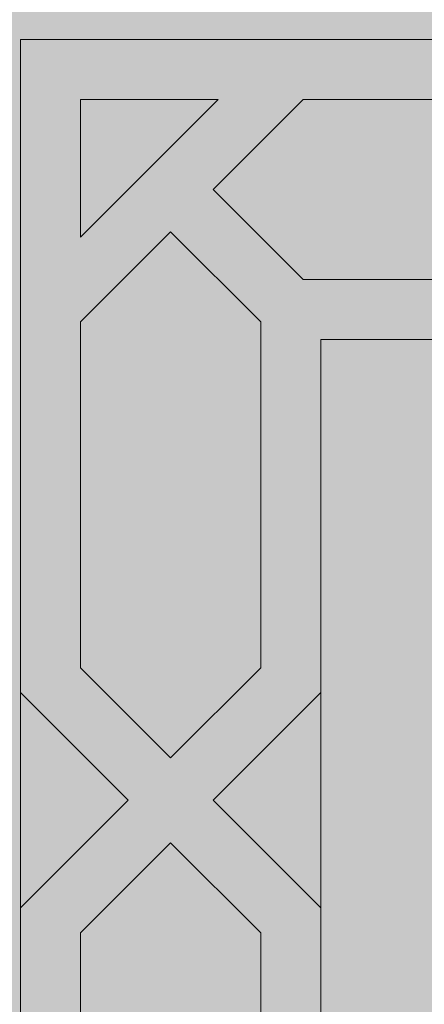
# Model space of a CAD drawing. Units: inches. Extents: x 844 to 2234, y 346 to 1084.
# Tile 81 of 93: x 1997.478 to 1999.197, y 708.742 to 712.926. Entities that reach past the tile are written whole.
import ezdxf

# ---------------------------------------------------------------- set-up
doc = ezdxf.new("R2010")
doc.units = ezdxf.units.IN
doc.header["$MEASUREMENT"] = 0
for name, color, linetype, lineweight in [('A-ANNO-DIMS', 2, 'Continuous', 18), ('furniture', 8, 'Continuous', 18), ('RA-AP-01$0$INT', 35, 'Continuous', 5)]:
    doc.layers.add(name, color=color, linetype=linetype, lineweight=lineweight)
doc.layers.add('RA-AP-01$0$FURN', color=3, linetype='Continuous')
doc.styles.get("Standard").update_dxf_attribs({"font": 'arial.ttf'})
doc.dimstyles.get("Standard").update_dxf_attribs({"dimtxt": 6, "dimasz": 3, "dimexe": 0.18, "dimexo": 0.0625, "dimgap": 0.09, "dimtad": 0, "dimtih": 1, "dimtoh": 1, "dimdec": 1, "dimzin": 0, "dimdsep": 46, "dimlunit": 3, "dimtxsty": 'Standard', "dimblk": 'ARCHTICK', "dimcen": 0.09, "dimadec": 0, "dimazin": 0, "dimtfac": 1, "dimtdec": 1, "dimtofl": 0, "dimtmove": 0, "dimatfit": 3, "dimfxl": 1, "dimtolj": 1, "dimtzin": 0, "dimarcsym": 0})

# ---------------------------------------------------------------- blocks, each defined once
blk = doc.blocks.new('A$C18D01794')
at = {"layer": 'RA-AP-01$0$INT'}
h = blk.add_hatch(color=256, dxfattribs=at)
h.paths.add_polyline_path([(4.355206456958071, -6.156712009588037), (4.355206456958071, -8.056712009588038), (5.455206456958072, -8.056712009588038), (5.455206456958072, -6.156712009588037)])
h.paths.add_polyline_path([(4.405206456958072, -8.006712009588039), (4.405206456958072, -6.206712009588038), (5.405206456958072, -6.206712009588038), (5.405206456958072, -8.006712009588039)], flags=16)
h = blk.add_hatch(color=256, dxfattribs=at)
h.paths.add_polyline_path([(4.505206456958071, -7.585498806127123), (4.46934859260189, -7.549640941759413), (4.505206456958071, -7.513783077414768), (4.505206456958071, -7.381963272220687), (4.469348592616735, -7.346105407867824), (4.505206456958071, -7.310247543514964), (4.505206456958071, -7.178427738324996), (4.469348592586679, -7.142569873965138), (4.505206456952245, -7.106712009588038), (4.476922185709333, -7.106712009588038), (4.455206456960671, -7.128427738343681), (4.433490728198047, -7.106712009588038), (4.405206456946033, -7.106712009588036), (4.441064321339216, -7.142569873969684), (4.40520645695807, -7.178427738362358), (4.405206456958072, -7.310247543472698), (4.441064321364728, -7.346105407867826), (4.40520645695807, -7.381963272262947), (4.40520645695807, -7.513783077378263), (4.441064321354429, -7.549640941786153), (4.405206456958072, -7.585498806170974), (4.405206456958072, -7.717318611286652), (4.441064321333084, -7.753176475673194), (4.405206456958072, -7.789034340036673), (4.405206456958072, -8.006712009588039), (4.644348592588106, -8.006712009588039), (4.680206456964639, -7.970854145211967), (4.716064321341165, -8.006712009588039), (4.869348592586113, -8.006712009588039), (4.905206456964143, -7.970854145210465), (4.941064321342174, -8.006712009588039), (5.094348592587118, -8.006712009588037), (5.130206456963649, -7.970854145211967), (5.166064321340178, -8.006712009588039), (5.405206456958072, -8.006712009588039), (5.405206456958072, -7.789034340024526), (5.369348592595202, -7.753176475673196), (5.40520645695807, -7.717318611298797), (5.40520645695807, -7.585498806158829), (5.369348592573859, -7.549640941786151), (5.40520645695807, -7.51378307739041), (5.40520645695807, -7.381963272250803), (5.36934859256356, -7.346105407867824), (5.405206456958072, -7.310247543484846), (5.405206456958072, -7.178427738350217), (5.369348592589068, -7.142569873969682), (5.405206456982249, -7.106712009588038), (5.376922185730244, -7.106712009588038), (5.355206456967613, -7.128427738343679), (5.333490728218955, -7.10671200958804), (5.305206456976043, -7.106712009588042), (5.341064321341609, -7.142569873965136), (5.305206456958072, -7.178427738337141), (5.305206456958072, -7.310247543502816), (5.34106432131155, -7.346105407867824), (5.305206456958072, -7.381963272232832), (5.30520645695807, -7.513783077402624), (5.341064321326395, -7.549640941759413), (5.305206456958072, -7.585498806139263), (5.305206456958072, -7.717318611299605), (5.341064321347738, -7.753176475677737), (5.305206456958072, -7.78903434007894), (5.30520645695807, -7.906712009588039), (5.166064321336834, -7.906712009588039), (5.130206456963647, -7.942569873961684), (5.094348592590464, -7.906712009588039), (4.941064321338827, -7.906712009588041), (4.905206456964145, -7.942569873963183), (4.869348592589459, -7.906712009588039), (4.716064321337822, -7.906712009588041), (4.680206456964641, -7.942569873961684), (4.644348592591453, -7.906712009588039), (4.505206456958071, -7.906712009588039), (4.505206456958071, -7.789034340066795), (4.469348592580545, -7.753176475677738), (4.505206456958071, -7.717318611311748)])
h.paths.add_polyline_path([(4.485206456974132, -7.709034340046354), (4.45520645695909, -7.739034340051736), (4.425206456974128, -7.709034340057131), (4.425206456993394, -7.593783077384998), (4.45520645699153, -7.563783077396511), (4.485206456993396, -7.593783077408017)], flags=16)
h.paths.add_polyline_path([(4.455206456954537, -7.767318611299197), (4.485206456958242, -7.797318611312542), (4.48520645695951, -7.912569873958716), (4.45520645695415, -7.942569873954422), (4.425206456957888, -7.912569873967813), (4.425206456957888, -7.797318611286197)], flags=16)
h.paths.add_polyline_path([(4.455206456964794, -7.535498806149051), (4.42520645696469, -7.5054988061393), (4.425206456983954, -7.390247543486406), (4.455206456990734, -7.360247543489279), (4.485206456983953, -7.39024754349214), (4.485206456964687, -7.505498806158811)], flags=16)
h.paths.add_polyline_path([(4.499348592588947, -7.926712009585049), (4.636064321340932, -7.926712009585049), (4.666064321342317, -7.956712009586821), (4.636064321343707, -7.986712009585048), (4.499348592575121, -7.986712009585048), (4.469348592591685, -7.956712009591957)], flags=16)
h.paths.add_polyline_path([(4.425206456957888, -7.940854145195974), (4.471064321332215, -7.986712009585049), (4.425206456957888, -7.986712009585049)], flags=16)
h.paths.add_polyline_path([(4.455206456990734, -7.331963272246367), (4.425206456989053, -7.301963272254337), (4.425206456969784, -7.186712009596224), (4.455206456965226, -7.156712009591144), (4.485206456969787, -7.186712009586051), (4.485206456989053, -7.301963272238404)], flags=16)
h.paths.add_polyline_path([(4.72434859258714, -7.926712009586255), (4.861064321340141, -7.926712009586248), (4.891064321340324, -7.956712009586823), (4.861064321340513, -7.986712009586252), (4.724348592586768, -7.986712009586252), (4.694348592586956, -7.956712009586821)], flags=16)
h.paths.add_polyline_path([(4.919348592587961, -7.956712009586821), (4.949348592588145, -7.92671200958625), (5.08606432134115, -7.926712009586253), (5.116064321341327, -7.956712009586823), (5.086064321341519, -7.986712009586252), (4.949348592587774, -7.986712009586252)], flags=16)
h.paths.add_polyline_path([(5.144348592585967, -7.956712009586823), (5.174348592587358, -7.926712009585049), (5.311064321339338, -7.926712009585049), (5.3410643213366, -7.956712009591957), (5.311064321353163, -7.986712009585048), (5.174348592584576, -7.986712009585048)], flags=16)
h.paths.add_polyline_path([(5.32520645693489, -7.593783077408021), (5.355206456936755, -7.563783077396511), (5.385206456934894, -7.593783077384998), (5.38520645695416, -7.709034340057128), (5.355206456969194, -7.739034340051736), (5.325206456954153, -7.709034340046352)], flags=16)
h.paths.add_polyline_path([(5.325206456970042, -7.797318611312542), (5.355206456973747, -7.767318611299197), (5.385206456970398, -7.7973186112862), (5.385206456970398, -7.912569873967816), (5.355206456974136, -7.942569873954422), (5.325206456968778, -7.912569873958716)], flags=16)
h.paths.add_polyline_path([(5.325206456963599, -7.505498806158811), (5.325206456944333, -7.39024754349214), (5.355206456937552, -7.360247543489279), (5.385206456944332, -7.39024754348641), (5.385206456963596, -7.505498806139303), (5.355206456963492, -7.53549880614905)], flags=16)
h.paths.add_polyline_path([(5.32520645693923, -7.301963272238403), (5.3252064569585, -7.186712009586051), (5.355206456963062, -7.156712009591142), (5.3852064569585, -7.186712009596224), (5.385206456939234, -7.301963272254338), (5.355206456937552, -7.331963272246369)], flags=16)
h.paths.add_polyline_path([(5.339348592596071, -7.986712009585048), (5.385206456970398, -7.940854145195972), (5.385206456970396, -7.986712009585048)], flags=16)
h = blk.add_hatch(color=256, dxfattribs=at)
h.paths.add_polyline_path([(4.469348592586677, -7.142569873965136), (4.505206456958073, -7.178427738324996), (4.505206456958071, -7.106712009582215)])
h.paths.add_polyline_path([(4.455206456960671, -7.128427738343681), (4.476922185709333, -7.106712009588038), (4.433490728198045, -7.106712009588038)])
h.paths.add_polyline_path([(4.405206456958073, -7.178427738362358), (4.441064321339218, -7.142569873969684), (4.40520645695807, -7.106712009600073)])
h.paths.add_polyline_path([(4.425206456989053, -7.301963272254335), (4.455206456990736, -7.331963272246371), (4.485206456989055, -7.301963272238399), (4.48520645696979, -7.186712009586054), (4.455206456965227, -7.15671200959114), (4.425206456969784, -7.186712009596224)])
h.paths.add_polyline_path([(4.505206456958073, -7.381963272220689), (4.505206456958071, -7.310247543514961), (4.469348592616738, -7.346105407867826)])
h.paths.add_polyline_path([(4.425206456964688, -7.5054988061393), (4.455206456964794, -7.535498806149051), (4.485206456964689, -7.505498806158811), (4.485206456983951, -7.390247543492138), (4.455206456990736, -7.360247543489277), (4.425206456983956, -7.39024754348641)])
h.paths.add_polyline_path([(4.425206456974126, -7.709034340057128), (4.455206456959092, -7.739034340051736), (4.485206456974132, -7.709034340046356), (4.485206456993396, -7.593783077408017), (4.45520645699153, -7.563783077396511), (4.425206456993394, -7.593783077384999)])
h.paths.add_polyline_path([(4.46934859260189, -7.549640941759415), (4.505206456958071, -7.585498806127123), (4.505206456958073, -7.513783077414766)])
h.paths.add_polyline_path([(4.405206456958073, -7.585498806170972), (4.441064321354427, -7.549640941786151), (4.405206456958072, -7.513783077378263)])
h.paths.add_polyline_path([(4.405206456958072, -7.789034340036673), (4.441064321333084, -7.753176475673194), (4.405206456958072, -7.71731861128665)])
h.paths.add_polyline_path([(4.469348592580547, -7.75317647567774), (4.505206456958071, -7.789034340066795), (4.505206456958071, -7.717318611311744)])
h.paths.add_polyline_path([(4.425206456957888, -7.912569873967814), (4.45520645695415, -7.942569873954422), (4.485206456959507, -7.912569873958718), (4.48520645695824, -7.797318611312542), (4.455206456954537, -7.767318611299197), (4.425206456957888, -7.797318611286202)])
h.paths.add_polyline_path([(4.425206456957888, -7.986712009585049), (4.471064321332215, -7.986712009585049), (4.425206456957888, -7.940854145195972)])
h.paths.add_polyline_path([(4.499348592575121, -7.986712009585048), (4.636064321343707, -7.986712009585049), (4.666064321342317, -7.956712009586823), (4.636064321340932, -7.926712009585049), (4.499348592588945, -7.926712009585049), (4.469348592591685, -7.95671200959196)])
h.paths.add_polyline_path([(4.680206456964641, -7.942569873961684), (4.716064321337824, -7.906712009588039), (4.644348592591454, -7.906712009588039)])
h.paths.add_polyline_path([(4.644348592588108, -8.006712009588039), (4.716064321341167, -8.006712009588039), (4.680206456964637, -7.970854145211964)])
h.paths.add_polyline_path([(4.724348592586768, -7.98671200958625), (4.861064321340514, -7.986712009586252), (4.891064321340324, -7.956712009586819), (4.861064321340141, -7.92671200958625), (4.724348592587134, -7.926712009586255), (4.694348592586957, -7.956712009586821)])
h.paths.add_polyline_path([(4.905206456964143, -7.942569873963183), (4.941064321338827, -7.906712009588039), (4.869348592589457, -7.906712009588037)])
h.paths.add_polyline_path([(4.869348592586113, -8.006712009588039), (4.941064321342172, -8.006712009588037), (4.905206456964145, -7.970854145210463)])
h.paths.add_polyline_path([(4.949348592587774, -7.986712009586252), (5.086064321341521, -7.986712009586252), (5.116064321341329, -7.956712009586823), (5.08606432134115, -7.926712009586253), (4.949348592588145, -7.92671200958625), (4.919348592587961, -7.956712009586819)])
h.paths.add_polyline_path([(5.130206456963645, -7.942569873961684), (5.166064321336834, -7.906712009588039), (5.094348592590464, -7.906712009588039)])
h.paths.add_polyline_path([(5.094348592587119, -8.006712009588039), (5.166064321340178, -8.006712009588039), (5.130206456963651, -7.970854145211967)])
h.paths.add_polyline_path([(5.174348592584578, -7.986712009585048), (5.311064321353163, -7.986712009585048), (5.341064321336602, -7.956712009591958), (5.31106432133934, -7.926712009585049), (5.174348592587352, -7.926712009585049), (5.144348592585969, -7.956712009586823)])
h.paths.add_polyline_path([(5.325206456968778, -7.912569873958718), (5.355206456974136, -7.942569873954422), (5.385206456970396, -7.912569873967814), (5.385206456970396, -7.797318611286199), (5.355206456973747, -7.767318611299197), (5.325206456970044, -7.797318611312544)])
h.paths.add_polyline_path([(5.339348592596073, -7.986712009585048), (5.385206456970396, -7.986712009585049), (5.385206456970398, -7.94085414519597)])
h.paths.add_polyline_path([(5.325206456954155, -7.709034340046354), (5.355206456969194, -7.739034340051734), (5.38520645695416, -7.709034340057128), (5.385206456934896, -7.593783077384999), (5.355206456936758, -7.563783077396513), (5.325206456934888, -7.593783077408019)])
h.paths.add_polyline_path([(5.305206456958072, -7.789034340078938), (5.341064321347739, -7.753176475677738), (5.305206456958072, -7.717318611299605)])
h.paths.add_polyline_path([(5.369348592595204, -7.753176475673194), (5.40520645695807, -7.789034340024526), (5.405206456958072, -7.717318611298798)])
h.paths.add_polyline_path([(5.405206456958072, -7.585498806158831), (5.405206456958072, -7.513783077390407), (5.369348592573857, -7.549640941786151)])
h.paths.add_polyline_path([(5.305206456958072, -7.585498806139266), (5.341064321326393, -7.549640941759413), (5.305206456958072, -7.513783077402626)])
h.paths.add_polyline_path([(5.325206456963599, -7.50549880615881), (5.355206456963494, -7.535498806149055), (5.385206456963598, -7.505498806139302), (5.385206456944334, -7.390247543486411), (5.355206456937552, -7.360247543489279), (5.325206456944333, -7.39024754349214)])
h.paths.add_polyline_path([(5.305206456958072, -7.38196327223283), (5.341064321311551, -7.346105407867824), (5.305206456958072, -7.31024754350282)])
h.paths.add_polyline_path([(5.325206456939231, -7.301963272238404), (5.355206456937552, -7.331963272246369), (5.385206456939235, -7.301963272254335), (5.385206456958502, -7.186712009596224), (5.355206456963061, -7.156712009591142), (5.3252064569585, -7.186712009586051)])
h.paths.add_polyline_path([(5.404581768715993, -7.381338584008926, -0.001217816984214), (5.405206456958072, -7.381112009582329), (5.405206456958072, -7.310247543484846), (5.369348592563558, -7.346105407867826)])
h.paths.add_polyline_path([(5.36934859258907, -7.142569873969684), (5.40520645695807, -7.178427738350215), (5.405206456958072, -7.106712009612218)])
h.paths.add_polyline_path([(5.355206456967613, -7.128427738343683), (5.376922185730239, -7.106712009588038), (5.333490728218953, -7.10671200958804)])
h.paths.add_polyline_path([(5.30520645695807, -7.178427738337139), (5.341064321341609, -7.142569873965134), (5.305206456958074, -7.10671200957007)])
blk.add_hatch(color=256, dxfattribs=at).paths.add_polyline_path([(4.505206456958071, -7.906712009588039), (5.305206456958072, -7.906712009588039), (5.305206456958072, -7.106712009588038), (5.255206456951893, -7.106712009588036), (5.25520645694868, -7.856712009570104), (4.555206456959269, -7.856712009588616), (4.555206456956052, -7.106712009588038), (4.505206456958073, -7.106712009588038)])
for p, q in [((5.32520645693489, -7.593783077408017), (5.325206456954155, -7.709034340046354)), ((5.385206456934892, -7.593783077384996), (5.385206456954159, -7.709034340057129)), ((5.325206456954155, -7.709034340046354), (5.355206456969194, -7.739034340051736)), ((5.385206456954159, -7.709034340057129), (5.355206456969194, -7.739034340051736)), ((5.305206456965273, -7.717318611306806), (5.341064321347739, -7.753176475677738)), ((5.405206456965273, -7.717318611291593), (5.369348592595202, -7.753176475673194)), ((5.341064321347739, -7.753176475677738), (5.305206456976345, -7.789034340060664)), ((5.369348592595202, -7.753176475673194), (5.40520645697813, -7.789034340044587)), ((5.355206456973749, -7.767318611299197), (5.325206456970044, -7.797318611312544)), ((5.355206456973749, -7.767318611299197), (5.385206456970398, -7.797318611286199)), ((5.325206456968778, -7.912569873958718), (5.325206456970044, -7.797318611312544)), ((5.385206456970398, -7.797318611286199), (5.385206456970398, -7.912569873967814)), ((5.325206456968778, -7.912569873958718), (5.355206456974136, -7.942569873954422)), ((5.385206456970398, -7.912569873967814), (5.355206456974136, -7.942569873954422)), ((5.174348592587354, -7.926712009585049), (5.31106432133934, -7.926712009585049)), ((5.31106432133934, -7.926712009585049), (5.341064321336602, -7.956712009591957)), ((5.339348592596073, -7.986712009585048), (5.385206456970398, -7.940854145195974)), ((5.385206456970398, -7.940854145195974), (5.385206456970398, -7.986712009585049)), ((5.311064321353163, -7.986712009585048), (5.341064321336602, -7.956712009591957)), ((5.174348592584578, -7.986712009585049), (5.311064321353163, -7.986712009585048)), ((5.339348592596073, -7.986712009585048), (5.385206456970398, -7.986712009585049))]:
    blk.add_line(p, q, dxfattribs=at)
for points in [[(5.405206456958072, -8.006712009588039), (4.405206456958072, -8.006712009588039), (4.405206456958072, -7.106712009588038)], [(5.305206456958072, -7.106712009588038), (5.305206456958072, -7.906712009588039), (4.505206456958071, -7.906712009588039), (4.505206456958071, -7.106712009588038)], [(5.405206456958072, -7.106712009588038), (5.405206456958072, -8.006712009588039)]]:
    blk.add_lwpolyline(points, dxfattribs=at)
blk = doc.blocks.new('A$C5D2F253E')
at = {"layer": 'RA-AP-01$0$FURN', "xscale": -0.7999999999883585, "yscale": 0.7999999999883585, "zscale": 0.8, "rotation": 90}
blk.add_blockref('A$C18D01794', (-5.687757199772477, 4.75791982714071), dxfattribs=at)
blk = doc.blocks.new('_ArchTick')
at = {"color": 0, "linetype": 'ByBlock', "const_width": 0.15}
blk.add_lwpolyline([(-0.5, -0.5), (0.5, 0.5)], dxfattribs=at)
blk = doc.blocks.new('*D121')
at = {"layer": 'A-ANNO-DIMS', "color": 0, "lineweight": -2, "transparency": 16777216}
for p, q in [((2030.271987351997, 734.262611118704), (2040.245275089302, 734.262611118704)), ((2040.065275089302, 734.262611118704), (2040.065275089302, 704.6043509484256)), ((2040.065275089302, 668.557359536674), (2040.065275089302, 698.2156197069523)), ((2030.271987351997, 668.557359536674), (2040.245275089302, 668.557359536674))]:
    blk.add_line(p, q, dxfattribs=at)
at = {"layer": 'Defpoints', "color": 0, "transparency": 16777216}
for p in [(2030.209487351997, 734.262611118704), (2040.065275089302, 734.262611118704), (2030.209487351997, 668.557359536674)]:
    blk.add_point(p, dxfattribs=at)
at = {"layer": 'A-ANNO-DIMS', "color": 0, "lineweight": -2, "transparency": 16777216, "xscale": 3, "yscale": 3, "zscale": 3}
for p, rotation in [((2040.065275089302, 734.262611118704), 90), ((2040.065275089302, 668.557359536674), 270)]:
    blk.add_blockref('_ArchTick', p, dxfattribs=dict(at, rotation=rotation))
at = {"layer": 'A-ANNO-DIMS', "color": 0, "transparency": 16777216, "insert": (2040.065275089302, 701.4099853276883), "char_height": 6, "attachment_point": 5}
blk.add_mtext('\\A1;LOUNGE SET 5\'-5 1/2" TYP.', dxfattribs=at)

msp = doc.modelspace()

# ---------------------------------------------------------------- block references
at = {"layer": 'furniture', "xscale": -15.94108302203742, "yscale": 15.94108302203742, "zscale": 15.94108302203742, "rotation": 270}
msp.add_blockref('A$C5D2F253E', (1990.567271852805, 701.4028671565849), dxfattribs=at)

# ---------------------------------------------------------------- dimensions: what is measured, and where the dimension line sits
at = {"layer": 'A-ANNO-DIMS'}
dim = msp.add_linear_dim(base=(2040.065275089302, 734.262611118704), p1=(2030.209487351996, 668.5573595366737), p2=(2030.209487351996, 734.2626111187037), angle=90, text='LOUNGE SET <> TYP.', dimstyle='Standard', override={"dimdec": 1, "dimlfac": 1, "dimrnd": 0, "dimzin": 1, "dimdsep": 46, "dimlunit": 4, "dimfrac": 2}, dxfattribs=at)
dim.commit()
dim.dimension.update_dxf_attribs({"geometry": '*D121', "text_midpoint": (2040.065275089302, 701.4099853276883)})

doc.saveas('drawing.dxf')
